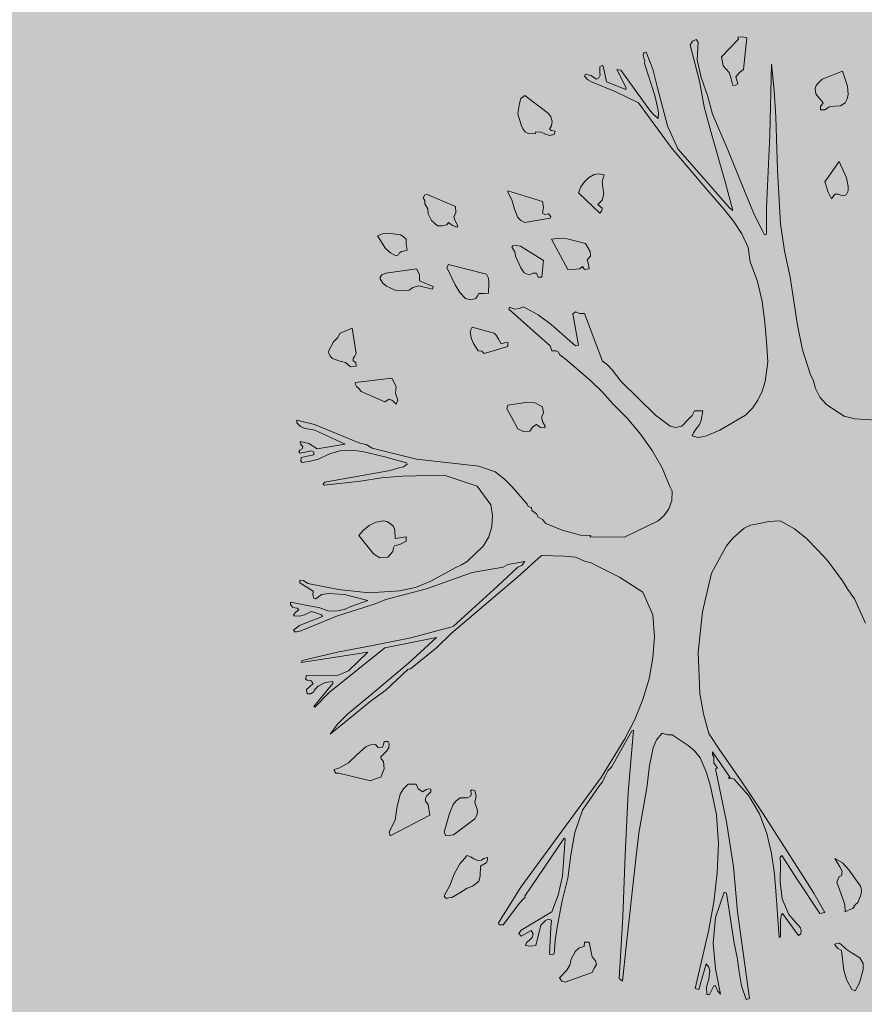
# Model space of a CAD drawing. Units: inches. Extents: x 84 to 1044, y -280 to 906.
# Tile 31 of 105: x 789 to 809, y -108 to -84. Entities that reach past the tile are written whole.
import ezdxf

# ---------------------------------------------------------------- set-up
doc = ezdxf.new("R2010")
doc.units = ezdxf.units.IN
doc.layers.add('L-PLNT', color=114, linetype='Continuous', lineweight=15)
doc.layers.add('L-PLNT-PATT', color=9, linetype='Continuous', lineweight=9, true_color=0xafd9aa)

# ---------------------------------------------------------------- blocks, each defined once
blk = doc.blocks.new('A$C37E508DF')
for p, q in [((0.6329, 1.5111), (0.6367, 1.5175)), ((0.6367, 1.5175), (0.6423, 1.5201)), ((0.6423, 1.5201), (0.6453, 1.5158)), ((0.6453, 1.5158), (0.644, 1.4879)), ((0.6826, 1.493), (0.7096, 1.5209)), ((0.7083, 1.5239), (0.7152, 1.5244)), ((0.7096, 1.5209), (0.7083, 1.5239)), ((0.7152, 1.5244), (0.7225, 1.5231)), ((0.7225, 1.5231), (0.7174, 1.4729)), ((0.5583, 1.4948), (0.5596, 1.4995)), ((0.5596, 1.4995), (0.563, 1.5003)), ((0.563, 1.5003), (0.5737, 1.4733)), ((0.6475, 1.4545), (0.6329, 1.5111)), ((0.5596, 1.4905), (0.5583, 1.4948)), ((0.5613, 1.4862), (0.5596, 1.4905)), ((0.5608, 1.4823), (0.5613, 1.4862)), ((0.5767, 1.4317), (0.5608, 1.4823)), ((0.644, 1.4879), (0.6505, 1.46)), ((0.6852, 1.4785), (0.6826, 1.493)), ((0.4897, 1.4772), (0.4935, 1.4789)), ((0.4897, 1.4678), (0.4897, 1.4772)), ((0.4905, 1.4635), (0.4897, 1.4678)), ((0.4935, 1.4789), (0.4952, 1.478)), ((0.4952, 1.478), (0.5004, 1.4532)), ((0.5313, 1.4437), (0.5167, 1.4729)), ((0.5167, 1.4729), (0.5231, 1.4716)), ((0.5231, 1.4716), (0.5686, 1.409)), ((0.5737, 1.4733), (0.5814, 1.4437)), ((0.6946, 1.4682), (0.6852, 1.4785)), ((0.6976, 1.4579), (0.6946, 1.4682)), ((0.7109, 1.4682), (0.7053, 1.4609)), ((0.7174, 1.4729), (0.7109, 1.4682)), ((0.7589, 1.3691), (0.7615, 1.481)), ((0.7615, 1.481), (0.7658, 1.4395)), ((0.8421, 1.4575), (0.8739, 1.4703)), ((0.8739, 1.4703), (0.882, 1.4463)), ((0.4657, 1.4622), (0.4669, 1.4652)), ((0.4708, 1.4566), (0.4657, 1.4622)), ((0.4669, 1.4652), (0.4755, 1.463)), ((0.4764, 1.4532), (0.4708, 1.4566)), ((0.4755, 1.463), (0.4845, 1.4575)), ((0.5154, 1.4373), (0.4764, 1.4532)), ((0.4845, 1.4575), (0.4884, 1.4596)), ((0.4884, 1.4596), (0.4905, 1.4635)), ((0.5004, 1.4532), (0.5308, 1.4412)), ((0.6552, 1.4137), (0.6475, 1.4545)), ((0.6505, 1.46), (0.6603, 1.4317)), ((0.7002, 1.4476), (0.6976, 1.4579)), ((0.7053, 1.4609), (0.7083, 1.4502)), ((0.8323, 1.4476), (0.8357, 1.451)), ((0.8357, 1.451), (0.8421, 1.4575)), ((0.551, 1.4197), (0.5154, 1.4373)), ((0.5308, 1.4412), (0.5313, 1.4437)), ((0.5814, 1.4437), (0.5969, 1.3833)), ((0.7049, 1.448), (0.7002, 1.4476)), ((0.7083, 1.4502), (0.7049, 1.448)), ((0.7658, 1.4395), (0.7684, 1.3979)), ((0.831, 1.4424), (0.8323, 1.4476)), ((0.8318, 1.4343), (0.831, 1.4424)), ((0.882, 1.4463), (0.8829, 1.433)), ((0.3628, 1.4189), (0.3649, 1.4266)), ((0.3649, 1.4266), (0.3709, 1.4317)), ((0.3709, 1.4317), (0.4086, 1.403)), ((0.6029, 1.3494), (0.551, 1.4197)), ((0.5814, 1.4133), (0.5767, 1.4317)), ((0.6603, 1.4317), (0.668, 1.4021)), ((0.8353, 1.4292), (0.8318, 1.4343)), ((0.8434, 1.4197), (0.8353, 1.4292)), ((0.8391, 1.4141), (0.8434, 1.4197)), ((0.8781, 1.4197), (0.8709, 1.4154)), ((0.8816, 1.4262), (0.8781, 1.4197)), ((0.8829, 1.433), (0.8816, 1.4262)), ((0.3598, 1.403), (0.3628, 1.4189)), ((0.5686, 1.409), (0.5741, 1.4021)), ((0.5827, 1.4043), (0.5814, 1.4133)), ((0.5823, 1.3953), (0.5827, 1.4043)), ((0.6655, 1.3743), (0.6552, 1.4137)), ((0.8395, 1.4086), (0.8391, 1.4141)), ((0.846, 1.4086), (0.8395, 1.4086)), ((0.8528, 1.4137), (0.846, 1.4086)), ((0.8619, 1.4146), (0.8528, 1.4137)), ((0.8709, 1.4154), (0.8619, 1.4146)), ((0.3602, 1.4021), (0.3598, 1.403)), ((0.364, 1.3888), (0.3602, 1.4021)), ((0.3657, 1.3828), (0.364, 1.3888)), ((0.4086, 1.403), (0.4125, 1.3979)), ((0.4125, 1.3979), (0.4142, 1.391)), ((0.4142, 1.391), (0.4134, 1.3837)), ((0.5741, 1.4021), (0.5823, 1.3953)), ((0.668, 1.4021), (0.6925, 1.3455)), ((0.7684, 1.3979), (0.771, 1.3134)), ((0.3683, 1.3781), (0.3657, 1.3828)), ((0.3718, 1.3738), (0.3683, 1.3781)), ((0.3765, 1.3713), (0.3718, 1.3738)), ((0.3885, 1.3738), (0.3872, 1.3708)), ((0.3971, 1.3734), (0.3885, 1.3738)), ((0.4039, 1.3704), (0.3971, 1.3734)), ((0.4134, 1.3837), (0.4099, 1.3781)), ((0.4099, 1.3781), (0.4134, 1.376)), ((0.4134, 1.376), (0.4189, 1.3751)), ((0.4189, 1.3751), (0.4176, 1.37)), ((0.5969, 1.3833), (0.6132, 1.3472)), ((0.6882, 1.2949), (0.6655, 1.3743)), ((0.3872, 1.3708), (0.3765, 1.3713)), ((0.4108, 1.3683), (0.4039, 1.3704)), ((0.4176, 1.37), (0.4108, 1.3683)), ((0.7538, 1.2529), (0.7589, 1.3691)), ((0.6595, 1.2829), (0.6029, 1.3494)), ((0.6132, 1.3472), (0.6959, 1.2529)), ((0.6925, 1.3455), (0.7161, 1.2868)), ((0.846, 1.2949), (0.8687, 1.3271)), ((0.8687, 1.3271), (0.8803, 1.3014)), ((0.771, 1.3134), (0.7761, 1.2285)), ((0.4597, 1.2868), (0.4648, 1.2945)), ((0.4648, 1.2945), (0.4717, 1.3009)), ((0.4717, 1.3009), (0.4807, 1.3065)), ((0.4807, 1.3065), (0.4884, 1.3074)), ((0.4884, 1.3074), (0.4965, 1.3057)), ((0.4965, 1.3057), (0.4935, 1.2954)), ((0.4935, 1.2954), (0.4948, 1.2855)), ((0.7002, 1.2495), (0.6882, 1.2949)), ((0.8473, 1.2924), (0.846, 1.2949)), ((0.8803, 1.3014), (0.8833, 1.2872)), ((0.3439, 1.2804), (0.3992, 1.2636)), ((0.3439, 1.2787), (0.3439, 1.2804)), ((0.4562, 1.2774), (0.4597, 1.2868)), ((0.4948, 1.2855), (0.4961, 1.2756)), ((0.6865, 1.2508), (0.6595, 1.2829)), ((0.7161, 1.2868), (0.7349, 1.2422)), ((0.8507, 1.2795), (0.8473, 1.2924)), ((0.8567, 1.2679), (0.8507, 1.2795)), ((0.8829, 1.2808), (0.8799, 1.2744)), ((0.8833, 1.2872), (0.8829, 1.2808)), ((0.2101, 1.2696), (0.2127, 1.2744)), ((0.2127, 1.2654), (0.2101, 1.2696)), ((0.2127, 1.2744), (0.2152, 1.2752)), ((0.2127, 1.2602), (0.2127, 1.2654)), ((0.2152, 1.2752), (0.2611, 1.2559)), ((0.3507, 1.2662), (0.3439, 1.2787)), ((0.3546, 1.2516), (0.3507, 1.2662)), ((0.3992, 1.2636), (0.4005, 1.2546)), ((0.4897, 1.2452), (0.4562, 1.2774)), ((0.4935, 1.2658), (0.4867, 1.2589)), ((0.4961, 1.2756), (0.4935, 1.2658)), ((0.8619, 1.2752), (0.8567, 1.2679)), ((0.867, 1.2752), (0.8619, 1.2752)), ((0.8713, 1.2739), (0.867, 1.2752)), ((0.8756, 1.2726), (0.8713, 1.2739)), ((0.8799, 1.2744), (0.8756, 1.2726)), ((0.2174, 1.2521), (0.2127, 1.2602)), ((0.2182, 1.2443), (0.2174, 1.2521)), ((0.2611, 1.2559), (0.262, 1.2465)), ((0.3602, 1.2383), (0.3546, 1.2516)), ((0.4005, 1.2546), (0.3992, 1.2452)), ((0.4867, 1.2589), (0.4935, 1.2529)), ((0.4931, 1.2491), (0.4897, 1.2452)), ((0.4935, 1.2529), (0.4931, 1.2491)), ((0.7015, 1.2323), (0.6865, 1.2508)), ((0.6959, 1.2529), (0.7002, 1.2495)), ((0.7538, 1.2122), (0.7538, 1.2529)), ((0.2234, 1.2336), (0.2182, 1.2443)), ((0.2328, 1.2251), (0.2234, 1.2336)), ((0.262, 1.2465), (0.2586, 1.2388)), ((0.2586, 1.2388), (0.2611, 1.2319)), ((0.3649, 1.2336), (0.3602, 1.2383)), ((0.3709, 1.2306), (0.3649, 1.2336)), ((0.4112, 1.2375), (0.3709, 1.2306)), ((0.3992, 1.2452), (0.4026, 1.2431)), ((0.4026, 1.2431), (0.4086, 1.2443)), ((0.4086, 1.2443), (0.4121, 1.2401)), ((0.4121, 1.2401), (0.4112, 1.2375)), ((0.7148, 1.2126), (0.7015, 1.2323)), ((0.7349, 1.2422), (0.7482, 1.216)), ((0.2401, 1.2251), (0.2328, 1.2251)), ((0.2474, 1.2268), (0.2401, 1.2251)), ((0.2504, 1.2306), (0.2474, 1.2268)), ((0.2568, 1.2255), (0.2504, 1.2306)), ((0.2633, 1.2229), (0.2568, 1.2255)), ((0.2611, 1.2319), (0.265, 1.2251)), ((0.265, 1.2251), (0.2633, 1.2229)), ((0.7761, 1.2285), (0.7821, 1.1856)), ((0.1376, 1.2092), (0.1458, 1.2126)), ((0.1389, 1.2079), (0.1376, 1.2092)), ((0.1505, 1.189), (0.1389, 1.2079)), ((0.1458, 1.2126), (0.1548, 1.2135)), ((0.1548, 1.2135), (0.1741, 1.2109)), ((0.1741, 1.2109), (0.1784, 1.2083)), ((0.1784, 1.2083), (0.1831, 1.204)), ((0.1831, 1.204), (0.1831, 1.1959)), ((0.4134, 1.204), (0.4258, 1.2058)), ((0.4391, 1.156), (0.4134, 1.204)), ((0.4258, 1.2058), (0.4382, 1.2045)), ((0.4382, 1.2045), (0.4669, 1.1972)), ((0.7246, 1.1908), (0.7148, 1.2126)), ((0.7482, 1.216), (0.7508, 1.2109)), ((0.7508, 1.2109), (0.7538, 1.2122)), ((0.1582, 1.1822), (0.1505, 1.189)), ((0.1788, 1.1852), (0.1758, 1.1847)), ((0.1848, 1.1865), (0.1788, 1.1852)), ((0.1831, 1.1959), (0.1848, 1.1865)), ((0.3507, 1.1916), (0.352, 1.1933)), ((0.355, 1.1839), (0.3507, 1.1916)), ((0.352, 1.1933), (0.3576, 1.1942)), ((0.3576, 1.1942), (0.364, 1.1929)), ((0.364, 1.1929), (0.4005, 1.1702)), ((0.4669, 1.1972), (0.4747, 1.1843)), ((0.7281, 1.168), (0.7246, 1.1908)), ((0.7821, 1.1856), (0.7911, 1.1436)), ((0.1668, 1.1775), (0.1582, 1.1822)), ((0.1711, 1.1792), (0.1668, 1.1775)), ((0.1728, 1.1826), (0.1711, 1.1792)), ((0.1758, 1.1847), (0.1728, 1.1826)), ((0.3563, 1.177), (0.355, 1.1839)), ((0.3645, 1.1586), (0.3563, 1.177)), ((0.4005, 1.1702), (0.3979, 1.1436)), ((0.4751, 1.177), (0.47, 1.1714)), ((0.47, 1.1714), (0.4721, 1.1646)), ((0.4747, 1.1843), (0.4751, 1.177)), ((0.1509, 1.1504), (0.1994, 1.1573)), ((0.1994, 1.1573), (0.2041, 1.1479)), ((0.2478, 1.1594), (0.2504, 1.1637)), ((0.2607, 1.1316), (0.2478, 1.1594)), ((0.2504, 1.1637), (0.3104, 1.1487)), ((0.37, 1.1509), (0.3645, 1.1586)), ((0.4519, 1.1564), (0.4391, 1.156)), ((0.458, 1.1573), (0.4519, 1.1564)), ((0.4622, 1.1607), (0.458, 1.1573)), ((0.4657, 1.156), (0.4622, 1.1607)), ((0.473, 1.1573), (0.4657, 1.156)), ((0.4721, 1.1646), (0.473, 1.1573)), ((0.7396, 1.1371), (0.7281, 1.168)), ((0.1419, 1.1436), (0.1449, 1.1474)), ((0.1419, 1.141), (0.1419, 1.1436)), ((0.1462, 1.1342), (0.1419, 1.141)), ((0.1449, 1.1474), (0.1509, 1.1504)), ((0.2041, 1.1479), (0.2045, 1.138)), ((0.3104, 1.1487), (0.3134, 1.1423)), ((0.3134, 1.1423), (0.3139, 1.1346)), ((0.3778, 1.1474), (0.37, 1.1509)), ((0.3842, 1.15), (0.3778, 1.1474)), ((0.3898, 1.15), (0.3842, 1.15)), ((0.3923, 1.1436), (0.3898, 1.15)), ((0.3979, 1.1436), (0.3923, 1.1436)), ((0.7911, 1.1436), (0.8027, 1.0677)), ((0.1522, 1.1294), (0.1462, 1.1342)), ((0.1655, 1.1234), (0.1522, 1.1294)), ((0.181, 1.1226), (0.1655, 1.1234)), ((0.1878, 1.1234), (0.181, 1.1226)), ((0.1938, 1.1273), (0.1878, 1.1234)), ((0.2032, 1.1303), (0.1938, 1.1273)), ((0.2247, 1.1251), (0.2032, 1.1303)), ((0.2045, 1.138), (0.226, 1.129)), ((0.226, 1.129), (0.2247, 1.1251)), ((0.268, 1.1196), (0.2607, 1.1316)), ((0.3139, 1.1346), (0.3134, 1.1183)), ((0.7469, 1.1054), (0.7396, 1.1371)), ((0.277, 1.1101), (0.268, 1.1196)), ((0.2856, 1.108), (0.277, 1.1101)), ((0.2933, 1.1101), (0.2856, 1.108)), ((0.2959, 1.1144), (0.2933, 1.1101)), ((0.2984, 1.1179), (0.2959, 1.1144)), ((0.3066, 1.1179), (0.2984, 1.1179)), ((0.3134, 1.1183), (0.3066, 1.1179)), ((0.3456, 1.093), (0.3469, 1.0964)), ((0.3842, 1.0591), (0.3456, 1.093)), ((0.3469, 1.0964), (0.355, 1.093)), ((0.355, 1.093), (0.3619, 1.0943)), ((0.3619, 1.0943), (0.3692, 1.0968)), ((0.3692, 1.0968), (0.3923, 1.0844)), ((0.7512, 1.0728), (0.7469, 1.1054)), ((0.3923, 1.0844), (0.4129, 1.069)), ((0.4472, 1.0857), (0.4515, 1.0887)), ((0.4562, 1.0364), (0.4472, 1.0857)), ((0.4515, 1.0887), (0.4584, 1.0865)), ((0.4584, 1.0865), (0.4657, 1.0861)), ((0.4657, 1.0861), (0.4939, 1.0107)), ((0.0789, 1.0552), (0.0978, 1.063)), ((0.0978, 1.063), (0.1042, 1.0231)), ((0.2847, 1.0565), (0.2856, 1.0604)), ((0.2856, 1.0604), (0.2877, 1.0647)), ((0.2877, 1.0647), (0.3224, 1.0552)), ((0.4129, 1.069), (0.4515, 1.0351)), ((0.7538, 1.0415), (0.7512, 1.0728)), ((0.8027, 1.0677), (0.8108, 1.0287)), ((0.0682, 1.0415), (0.0746, 1.0475)), ((0.0746, 1.0475), (0.0789, 1.0552)), ((0.2851, 1.054), (0.2847, 1.0565)), ((0.2864, 1.0463), (0.2851, 1.054)), ((0.2899, 1.039), (0.2864, 1.0463)), ((0.3224, 1.0552), (0.3255, 1.0522)), ((0.3255, 1.0522), (0.3293, 1.0458)), ((0.3293, 1.0458), (0.3336, 1.0381)), ((0.4112, 1.0351), (0.3842, 1.0591)), ((0.0596, 1.0257), (0.0682, 1.0415)), ((0.2972, 1.0274), (0.2899, 1.039)), ((0.3439, 1.0338), (0.3066, 1.0231)), ((0.3336, 1.0381), (0.3383, 1.0398)), ((0.3383, 1.0398), (0.3439, 1.0402)), ((0.3439, 1.0402), (0.3439, 1.0338)), ((0.4138, 1.0274), (0.4112, 1.0351)), ((0.4515, 1.0351), (0.4562, 1.0364)), ((0.7559, 1.0098), (0.7538, 1.0415)), ((0.0626, 1.0188), (0.0596, 1.0257)), ((0.0665, 1.0149), (0.0626, 1.0188)), ((0.0763, 1.0111), (0.0665, 1.0149)), ((0.1012, 1.018), (0.099, 1.0149)), ((0.099, 1.0149), (0.099, 1.0111)), ((0.1042, 1.0231), (0.1012, 1.018)), ((0.3032, 1.0265), (0.2972, 1.0274)), ((0.3066, 1.0231), (0.3032, 1.0265)), ((0.4202, 1.0274), (0.4138, 1.0274)), ((0.4241, 1.0257), (0.4202, 1.0274)), ((0.4267, 1.0209), (0.4241, 1.0257)), ((0.4305, 1.0175), (0.4267, 1.0209)), ((0.4378, 1.0124), (0.4305, 1.0175)), ((0.8108, 1.0287), (0.8233, 0.9892)), ((0.087, 1.0085), (0.0763, 1.0111)), ((0.0948, 1.0016), (0.087, 1.0085)), ((0.1042, 1.0029), (0.0948, 1.0016)), ((0.099, 1.0111), (0.1033, 1.0085)), ((0.1033, 1.0085), (0.1042, 1.0029)), ((0.476, 0.9789), (0.4378, 1.0124)), ((0.4939, 1.0107), (0.5021, 1.0051)), ((0.5021, 1.0051), (0.5094, 0.9969)), ((0.7516, 0.9785), (0.7559, 1.0098)), ((0.1029, 0.9772), (0.1604, 0.9841)), ((0.1604, 0.9841), (0.1672, 0.9708)), ((0.5094, 0.9969), (0.5231, 0.9789)), ((0.8233, 0.9892), (0.8275, 0.9815)), ((0.1025, 0.9751), (0.1029, 0.9772)), ((0.1046, 0.9708), (0.1025, 0.9751)), ((0.1076, 0.9682), (0.1046, 0.9708)), ((0.1119, 0.9626), (0.1076, 0.9682)), ((0.1672, 0.9708), (0.1664, 0.9601)), ((0.4939, 0.9618), (0.476, 0.9789)), ((0.5231, 0.9789), (0.578, 0.9253)), ((0.7469, 0.9635), (0.7516, 0.9785)), ((0.8275, 0.9815), (0.8314, 0.9673)), ((0.8314, 0.9673), (0.8383, 0.954)), ((0.1496, 0.9463), (0.1119, 0.9626)), ((0.1664, 0.9601), (0.1698, 0.9493)), ((0.5111, 0.9429), (0.4939, 0.9618)), ((0.7401, 0.9493), (0.7469, 0.9635)), ((0.8383, 0.954), (0.8486, 0.942)), ((0.1565, 0.9506), (0.1496, 0.9463)), ((0.1604, 0.9493), (0.1565, 0.9506)), ((0.1629, 0.9468), (0.1604, 0.9493)), ((0.1672, 0.9429), (0.1629, 0.9468)), ((0.1698, 0.9493), (0.1672, 0.9429)), ((0.3426, 0.936), (0.3443, 0.9412)), ((0.3602, 0.9039), (0.3426, 0.936)), ((0.3443, 0.9412), (0.3722, 0.9451)), ((0.3722, 0.9451), (0.3868, 0.9446)), ((0.3868, 0.9446), (0.3992, 0.9386)), ((0.3992, 0.9386), (0.4009, 0.9292)), ((0.5334, 0.9202), (0.5111, 0.9429)), ((0.7203, 0.9253), (0.7315, 0.9365)), ((0.7315, 0.9365), (0.7401, 0.9493)), ((0.8486, 0.942), (0.8619, 0.933)), ((0.4009, 0.9292), (0.3975, 0.9215)), ((0.3975, 0.9215), (0.3996, 0.9142)), ((0.554, 0.8953), (0.5334, 0.9202)), ((0.578, 0.9253), (0.6011, 0.9077)), ((0.6303, 0.9189), (0.6359, 0.9245)), ((0.6359, 0.9245), (0.6397, 0.9322)), ((0.6397, 0.9322), (0.653, 0.9322)), ((0.653, 0.9322), (0.6505, 0.9172)), ((0.6796, 0.9013), (0.7203, 0.9253)), ((0.8619, 0.933), (0.8769, 0.9236)), ((0.8769, 0.9236), (0.8936, 0.9193)), ((0.0103, 0.9129), (0.0103, 0.9172)), ((0.0103, 0.9172), (0.0382, 0.9107)), ((0.0159, 0.9073), (0.0103, 0.9129)), ((0.0232, 0.9043), (0.0159, 0.9073)), ((0.0382, 0.9107), (0.1098, 0.8807)), ((0.3838, 0.9069), (0.379, 0.9)), ((0.3898, 0.9107), (0.3838, 0.9069)), ((0.3958, 0.906), (0.3898, 0.9107)), ((0.4026, 0.9052), (0.3958, 0.906)), ((0.3996, 0.9142), (0.4031, 0.9077)), ((0.4031, 0.9077), (0.4026, 0.9052)), ((0.6011, 0.9077), (0.6097, 0.9056)), ((0.6097, 0.9056), (0.6196, 0.9077)), ((0.6196, 0.9077), (0.6303, 0.9189)), ((0.6479, 0.9103), (0.6423, 0.9039)), ((0.6505, 0.9172), (0.6479, 0.9103)), ((0.8936, 0.9193), (0.9279, 0.9172)), ((0.0386, 0.9013), (0.0232, 0.9043)), ((0.0866, 0.8794), (0.0386, 0.9013)), ((0.3692, 0.8992), (0.3602, 0.9039)), ((0.379, 0.9), (0.3692, 0.8992)), ((0.5728, 0.8691), (0.554, 0.8953)), ((0.6384, 0.8974), (0.6359, 0.8927)), ((0.6359, 0.8927), (0.6457, 0.8897)), ((0.6423, 0.9039), (0.6384, 0.8974)), ((0.6457, 0.8897), (0.6569, 0.8919)), ((0.6569, 0.8919), (0.6796, 0.9013)), ((0.0159, 0.8803), (0.0154, 0.8837)), ((0.0154, 0.8837), (0.0292, 0.8803)), ((0.0176, 0.8777), (0.0159, 0.8803)), ((0.0193, 0.8752), (0.0176, 0.8777)), ((0.0184, 0.8717), (0.0193, 0.8752)), ((0.0292, 0.8803), (0.0424, 0.8717)), ((0.0424, 0.8717), (0.0866, 0.8794)), ((0.1098, 0.8807), (0.1196, 0.8786)), ((0.1196, 0.8786), (0.1295, 0.873)), ((0.0133, 0.8679), (0.015, 0.87)), ((0.0154, 0.8649), (0.0133, 0.8679)), ((0.015, 0.87), (0.0184, 0.8717)), ((0.0334, 0.8687), (0.0154, 0.8649)), ((0.0163, 0.8529), (0.0171, 0.8584)), ((0.0171, 0.8584), (0.0266, 0.8602)), ((0.0266, 0.8602), (0.0369, 0.8623)), ((0.0369, 0.8666), (0.0334, 0.8687)), ((0.0369, 0.8623), (0.0369, 0.8666)), ((0.0617, 0.864), (0.0442, 0.8554)), ((0.0789, 0.8687), (0.0617, 0.864)), ((0.0965, 0.8696), (0.0789, 0.8687)), ((0.1141, 0.8679), (0.0965, 0.8696)), ((0.1492, 0.8593), (0.1141, 0.8679)), ((0.1295, 0.873), (0.1994, 0.8554)), ((0.1835, 0.8499), (0.1492, 0.8593)), ((0.5887, 0.8421), (0.5728, 0.8691)), ((0.0184, 0.8503), (0.0163, 0.8529)), ((0.0317, 0.8524), (0.0184, 0.8503)), ((0.0442, 0.8554), (0.0317, 0.8524)), ((0.1698, 0.8413), (0.1792, 0.8434)), ((0.1792, 0.8434), (0.1848, 0.8477)), ((0.1848, 0.8477), (0.1835, 0.8499)), ((0.1994, 0.8554), (0.2984, 0.8447)), ((0.2984, 0.8447), (0.3242, 0.8357)), ((0.6007, 0.8125), (0.5887, 0.8421)), ((0.0545, 0.8194), (0.1578, 0.8378)), ((0.1771, 0.8288), (0.1441, 0.8258)), ((0.1578, 0.8378), (0.1698, 0.8413)), ((0.2436, 0.8301), (0.1771, 0.8288)), ((0.2954, 0.813), (0.2436, 0.8301)), ((0.3242, 0.8357), (0.3387, 0.8241)), ((0.0519, 0.8164), (0.0545, 0.8194)), ((0.0532, 0.8143), (0.0519, 0.8164)), ((0.1111, 0.8207), (0.0532, 0.8143)), ((0.1441, 0.8258), (0.1111, 0.8207)), ((0.3173, 0.7834), (0.2954, 0.813)), ((0.3387, 0.8241), (0.3512, 0.8117)), ((0.3512, 0.8117), (0.3748, 0.7842)), ((0.6046, 0.8048), (0.6007, 0.8125)), ((0.6037, 0.7903), (0.6046, 0.8048)), ((0.3199, 0.7662), (0.3173, 0.7834)), ((0.3748, 0.7842), (0.3765, 0.7804)), ((0.3765, 0.7804), (0.3816, 0.7791)), ((0.599, 0.777), (0.6037, 0.7903)), ((0.3186, 0.7491), (0.3199, 0.7662)), ((0.3816, 0.7791), (0.382, 0.7744)), ((0.382, 0.7744), (0.3859, 0.7714)), ((0.3859, 0.7714), (0.3902, 0.7684)), ((0.3902, 0.7684), (0.3919, 0.7641)), ((0.5823, 0.7577), (0.5913, 0.7658)), ((0.5913, 0.7658), (0.599, 0.777)), ((0.1153, 0.7427), (0.1244, 0.7504)), ((0.1244, 0.7504), (0.1351, 0.7559)), ((0.1351, 0.7559), (0.1471, 0.7577)), ((0.1471, 0.7577), (0.1527, 0.7568)), ((0.1527, 0.7568), (0.1578, 0.7538)), ((0.1578, 0.7538), (0.1629, 0.7491)), ((0.1629, 0.7491), (0.1651, 0.7431)), ((0.3139, 0.7324), (0.3186, 0.7491)), ((0.3919, 0.7641), (0.3988, 0.7598)), ((0.3988, 0.7598), (0.4043, 0.7538)), ((0.4043, 0.7538), (0.4301, 0.7431)), ((0.5287, 0.7319), (0.5823, 0.7577)), ((0.7285, 0.7512), (0.7182, 0.7461)), ((0.7401, 0.7534), (0.7285, 0.7512)), ((0.7577, 0.7568), (0.7401, 0.7534)), ((0.7752, 0.7577), (0.7577, 0.7568)), ((0.798, 0.7452), (0.7752, 0.7577)), ((0.1081, 0.7349), (0.1153, 0.7427)), ((0.1312, 0.7058), (0.1081, 0.7349)), ((0.1651, 0.7431), (0.1655, 0.7298)), ((0.4301, 0.7431), (0.4515, 0.7371)), ((0.4515, 0.7371), (0.4635, 0.7341)), ((0.4635, 0.7341), (0.4755, 0.7349)), ((0.4755, 0.7349), (0.4742, 0.7324)), ((0.7182, 0.7461), (0.7002, 0.7307)), ((0.8173, 0.7298), (0.798, 0.7452)), ((0.1646, 0.7186), (0.1629, 0.7152)), ((0.1741, 0.7208), (0.1646, 0.7186)), ((0.1655, 0.7298), (0.1831, 0.7324)), ((0.1831, 0.7255), (0.1741, 0.7208)), ((0.1831, 0.7324), (0.1831, 0.7255)), ((0.28, 0.6933), (0.3049, 0.7178)), ((0.3049, 0.7178), (0.3139, 0.7324)), ((0.4742, 0.7324), (0.5287, 0.7319)), ((0.6903, 0.7186), (0.6818, 0.7032)), ((0.7002, 0.7307), (0.6903, 0.7186)), ((0.8344, 0.7122), (0.8173, 0.7298)), ((0.1415, 0.6994), (0.1312, 0.7058)), ((0.1621, 0.7092), (0.1539, 0.7002)), ((0.1629, 0.7152), (0.1621, 0.7092)), ((0.3975, 0.7028), (0.3598, 0.6693)), ((0.4339, 0.7019), (0.3975, 0.7028)), ((0.4515, 0.7002), (0.4339, 0.7019)), ((0.6818, 0.7032), (0.6667, 0.6749)), ((0.8503, 0.6951), (0.8344, 0.7122)), ((0.1539, 0.7002), (0.1415, 0.6994)), ((0.262, 0.6839), (0.271, 0.6882)), ((0.271, 0.6882), (0.28, 0.6933)), ((0.3443, 0.6886), (0.337, 0.6843)), ((0.3533, 0.6903), (0.3443, 0.6886)), ((0.3709, 0.6933), (0.3533, 0.6903)), ((0.3598, 0.6843), (0.3662, 0.6873)), ((0.3662, 0.6873), (0.3709, 0.6933)), ((0.4674, 0.6933), (0.4515, 0.7002)), ((0.476, 0.6912), (0.4674, 0.6933)), ((0.4832, 0.6878), (0.476, 0.6912)), ((0.521, 0.6685), (0.4832, 0.6878)), ((0.8739, 0.6629), (0.8503, 0.6951)), ((0.2877, 0.6762), (0.2152, 0.6505)), ((0.2221, 0.6625), (0.262, 0.6839)), ((0.337, 0.6843), (0.2877, 0.6762)), ((0.328, 0.6543), (0.3598, 0.6843)), ((0.6667, 0.6749), (0.6526, 0.614)), ((0.0146, 0.6599), (0.0146, 0.6642)), ((0.0146, 0.6642), (0.0206, 0.6633)), ((0.036, 0.6466), (0.0146, 0.6599)), ((0.0206, 0.6633), (0.0274, 0.6586)), ((0.0274, 0.6586), (0.0759, 0.6492)), ((0.1977, 0.6526), (0.2221, 0.6625)), ((0.3598, 0.6693), (0.2543, 0.5797)), ((0.5578, 0.6449), (0.521, 0.6685)), ((0.8824, 0.6492), (0.8739, 0.6629)), ((0.0356, 0.6406), (0.036, 0.6466)), ((0.0369, 0.6355), (0.0356, 0.6406)), ((0.0489, 0.641), (0.0399, 0.6342)), ((0.0609, 0.6428), (0.0489, 0.641)), ((0.0853, 0.641), (0.0609, 0.6428)), ((0.0759, 0.6492), (0.1244, 0.644)), ((0.1226, 0.632), (0.0853, 0.641)), ((0.1244, 0.644), (0.1728, 0.647)), ((0.2152, 0.6505), (0.1509, 0.6333)), ((0.1728, 0.647), (0.1977, 0.6526)), ((0.2581, 0.5913), (0.328, 0.6543)), ((0.5737, 0.6089), (0.5578, 0.6449)), ((0.8932, 0.6342), (0.8824, 0.6492)), ((0, 0.629), (0.0467, 0.62)), ((0, 0.6252), (0, 0.629)), ((0.003, 0.6213), (0, 0.6252)), ((0.0399, 0.6342), (0.0369, 0.6355)), ((0.0973, 0.6226), (0.1226, 0.632)), ((0.1342, 0.6265), (0.1175, 0.6213)), ((0.1509, 0.6333), (0.1342, 0.6265)), ((0.9103, 0.5956), (0.8932, 0.6342)), ((0.0069, 0.6204), (0.003, 0.6213)), ((0.0047, 0.6093), (0.0086, 0.6132)), ((0.0056, 0.6076), (0.0047, 0.6093)), ((0.0107, 0.6196), (0.0069, 0.6204)), ((0.0086, 0.6132), (0.0133, 0.617)), ((0.0133, 0.617), (0.0107, 0.6196)), ((0.0223, 0.6089), (0.0141, 0.6072)), ((0.0334, 0.6145), (0.0223, 0.6089)), ((0.0416, 0.6119), (0.0334, 0.6145)), ((0.0493, 0.6093), (0.0416, 0.6119)), ((0.0467, 0.62), (0.0592, 0.6153)), ((0.0506, 0.6063), (0.0493, 0.6093)), ((0.0592, 0.6153), (0.072, 0.6149)), ((0.072, 0.6149), (0.0849, 0.6175)), ((0.1175, 0.6213), (0.0746, 0.6076)), ((0.0849, 0.6175), (0.0973, 0.6226)), ((0.5763, 0.5741), (0.5737, 0.6089)), ((0.6526, 0.614), (0.6457, 0.5497)), ((0.0141, 0.6072), (0.0056, 0.6076)), ((0.0141, 0.5921), (0.0257, 0.5969)), ((0.0746, 0.6076), (0.0163, 0.5836)), ((0.0257, 0.5969), (0.0506, 0.6063)), ((0.0047, 0.5849), (0.0141, 0.5921)), ((0.0069, 0.5823), (0.0047, 0.5849)), ((0.0099, 0.5823), (0.0069, 0.5823)), ((0.0163, 0.5836), (0.0099, 0.5823)), ((0.1904, 0.5724), (0.2474, 0.5879)), ((0.2543, 0.5797), (0.2311, 0.557)), ((0.2474, 0.5879), (0.253, 0.5892)), ((0.253, 0.5892), (0.2581, 0.5913)), ((0.1325, 0.5608), (0.1904, 0.5724)), ((0.2311, 0.5729), (0.1496, 0.557)), ((0.1869, 0.5325), (0.2311, 0.5729)), ((0.5737, 0.5407), (0.5763, 0.5741)), ((0.1226, 0.5497), (0.0171, 0.5338)), ((0.0184, 0.5368), (0.0746, 0.5501)), ((0.1496, 0.557), (0.0613, 0.4858)), ((0.0746, 0.5501), (0.1325, 0.5608)), ((0.0917, 0.5205), (0.1226, 0.5497)), ((0.2311, 0.557), (0.1899, 0.5235)), ((0.6457, 0.5497), (0.6483, 0.4845)), ((0.0171, 0.5338), (0.0184, 0.5368)), ((0.1269, 0.482), (0.1869, 0.5325)), ((0.5677, 0.5077), (0.5737, 0.5407)), ((0.0755, 0.5133), (0.0917, 0.5205)), ((0.1861, 0.5231), (0.1509, 0.4897)), ((0.1899, 0.5235), (0.1861, 0.5231)), ((0.024, 0.5072), (0.0253, 0.5128)), ((0.0262, 0.5055), (0.024, 0.5072)), ((0.0253, 0.5128), (0.042, 0.5133)), ((0.0326, 0.5047), (0.0262, 0.5055)), ((0.03, 0.4948), (0.036, 0.5004)), ((0.036, 0.5004), (0.0326, 0.5047)), ((0.0369, 0.4639), (0.0669, 0.5004)), ((0.042, 0.5133), (0.0587, 0.5124)), ((0.0549, 0.5021), (0.0437, 0.4961)), ((0.0669, 0.5034), (0.0549, 0.5021)), ((0.0587, 0.5124), (0.0755, 0.5133)), ((0.0669, 0.5004), (0.0669, 0.5034)), ((0.5578, 0.4751), (0.5677, 0.5077)), ((0.0253, 0.491), (0.03, 0.4948)), ((0.0262, 0.4841), (0.0253, 0.491)), ((0.0317, 0.4841), (0.0262, 0.4841)), ((0.0369, 0.4871), (0.0317, 0.4841)), ((0.0382, 0.4905), (0.0369, 0.4871)), ((0.0403, 0.4922), (0.0382, 0.4905)), ((0.0613, 0.4858), (0.0386, 0.4627)), ((0.0437, 0.4961), (0.0403, 0.4922)), ((0.1509, 0.4897), (0.1282, 0.4734)), ((0.6483, 0.4845), (0.6539, 0.4524)), ((0.1282, 0.4734), (0.0626, 0.4198)), ((0.0905, 0.4515), (0.1269, 0.482)), ((0.545, 0.4434), (0.5578, 0.4751)), ((0.0386, 0.4627), (0.0369, 0.4639)), ((0.6539, 0.4524), (0.6625, 0.4211)), ((0.0746, 0.4361), (0.0905, 0.4515)), ((0.5295, 0.4125), (0.545, 0.4434)), ((0.0626, 0.4198), (0.0746, 0.4361)), ((0.5403, 0.4254), (0.5081, 0.3679)), ((0.5347, 0.3276), (0.5433, 0.4266)), ((0.5433, 0.4266), (0.5403, 0.4254)), ((0.5887, 0.4215), (0.5797, 0.4112)), ((0.5969, 0.4189), (0.5887, 0.4215)), ((0.6625, 0.4211), (0.6796, 0.3945)), ((0.1471, 0.4035), (0.1484, 0.4082)), ((0.1484, 0.4082), (0.1548, 0.4082)), ((0.1548, 0.4082), (0.1565, 0.4052)), ((0.4922, 0.3516), (0.5295, 0.4125)), ((0.5797, 0.4112), (0.5741, 0.3983)), ((0.6046, 0.4189), (0.5969, 0.4189)), ((0.6295, 0.4022), (0.6046, 0.4189)), ((0.1055, 0.388), (0.1192, 0.4001)), ((0.1192, 0.4001), (0.1265, 0.4031)), ((0.1265, 0.4031), (0.1346, 0.4039)), ((0.1346, 0.4039), (0.1389, 0.3992)), ((0.1389, 0.3992), (0.1458, 0.3996)), ((0.1518, 0.3932), (0.1432, 0.3842)), ((0.1458, 0.3996), (0.1471, 0.4035)), ((0.1556, 0.3983), (0.1518, 0.3932)), ((0.1565, 0.4052), (0.1556, 0.3983)), ((0.5741, 0.3983), (0.5686, 0.3705)), ((0.6397, 0.3936), (0.6295, 0.4022)), ((0.6487, 0.3825), (0.6397, 0.3936)), ((0.6959, 0.352), (0.668, 0.3919)), ((0.668, 0.3919), (0.668, 0.3872)), ((0.6796, 0.3945), (0.7148, 0.3447)), ((0.0763, 0.3662), (0.0917, 0.3748)), ((0.0917, 0.3748), (0.1055, 0.388)), ((0.1432, 0.3842), (0.1436, 0.3808)), ((0.1436, 0.3808), (0.1471, 0.3769)), ((0.1471, 0.3769), (0.1484, 0.3649)), ((0.6582, 0.3602), (0.6487, 0.3825)), ((0.668, 0.3872), (0.6706, 0.3842)), ((0.6706, 0.3842), (0.6702, 0.3748)), ((0.6702, 0.3748), (0.6762, 0.3662)), ((0.069, 0.364), (0.0763, 0.3662)), ((0.069, 0.3627), (0.069, 0.364)), ((0.0716, 0.3585), (0.069, 0.3627)), ((0.1484, 0.3649), (0.1432, 0.352)), ((0.5025, 0.3619), (0.4982, 0.3537)), ((0.5081, 0.3679), (0.5025, 0.3619)), ((0.5686, 0.3705), (0.5643, 0.3349)), ((0.665, 0.3379), (0.6582, 0.3602)), ((0.6762, 0.3662), (0.6732, 0.3653)), ((0.6732, 0.3653), (0.6903, 0.2813)), ((0.0763, 0.3585), (0.0716, 0.3585)), ((0.1269, 0.3464), (0.0763, 0.3585)), ((0.1355, 0.3499), (0.1269, 0.3464)), ((0.1432, 0.352), (0.1355, 0.3499)), ((0.4065, 0.2345), (0.4922, 0.3516)), ((0.4939, 0.3447), (0.4884, 0.337)), ((0.4982, 0.3537), (0.4939, 0.3447)), ((0.6933, 0.3503), (0.6959, 0.352)), ((0.6985, 0.3503), (0.6933, 0.3503)), ((0.7023, 0.349), (0.6985, 0.3503)), ((0.7259, 0.3224), (0.7023, 0.349)), ((0.7148, 0.3447), (0.7487, 0.2937)), ((0.1737, 0.325), (0.1788, 0.3336)), ((0.1788, 0.3336), (0.1861, 0.3409)), ((0.1861, 0.3409), (0.199, 0.3409)), ((0.199, 0.3409), (0.2024, 0.3336)), ((0.2024, 0.3336), (0.2097, 0.3289)), ((0.2097, 0.3289), (0.2148, 0.3323)), ((0.2148, 0.3323), (0.2182, 0.3336)), ((0.2221, 0.3289), (0.2161, 0.3224)), ((0.2182, 0.3336), (0.2221, 0.3327)), ((0.2221, 0.3327), (0.2221, 0.3289)), ((0.2851, 0.3302), (0.2877, 0.3319)), ((0.2864, 0.325), (0.2851, 0.3302)), ((0.2877, 0.3319), (0.292, 0.3306)), ((0.292, 0.3306), (0.2941, 0.322)), ((0.4884, 0.337), (0.4622, 0.2997)), ((0.53, 0.229), (0.5347, 0.3276)), ((0.5643, 0.3349), (0.5578, 0.2993)), ((0.6745, 0.2924), (0.665, 0.3379)), ((0.1689, 0.3053), (0.1737, 0.325)), ((0.2161, 0.3224), (0.214, 0.3186)), ((0.214, 0.3186), (0.214, 0.3139)), ((0.214, 0.3139), (0.2182, 0.3087)), ((0.2577, 0.3087), (0.2624, 0.3147)), ((0.2624, 0.3147), (0.2689, 0.3194)), ((0.2689, 0.3194), (0.2796, 0.3194)), ((0.2796, 0.3194), (0.2847, 0.3211)), ((0.2847, 0.3211), (0.2864, 0.325)), ((0.2941, 0.322), (0.292, 0.3117)), ((0.7427, 0.2937), (0.7259, 0.3224)), ((0.1655, 0.2843), (0.1689, 0.3053)), ((0.2182, 0.3087), (0.2204, 0.292)), ((0.2517, 0.2946), (0.2577, 0.3087)), ((0.292, 0.3117), (0.2959, 0.2993)), ((0.2959, 0.2993), (0.2954, 0.2928)), ((0.4622, 0.2997), (0.4502, 0.2645)), ((0.5578, 0.2993), (0.5518, 0.2633)), ((0.1565, 0.265), (0.1655, 0.2843)), ((0.2204, 0.292), (0.1578, 0.259)), ((0.2436, 0.265), (0.2517, 0.2946)), ((0.292, 0.286), (0.2581, 0.2607)), ((0.2954, 0.2928), (0.292, 0.286)), ((0.6775, 0.2465), (0.6745, 0.2924)), ((0.6903, 0.2813), (0.7015, 0.2101)), ((0.7542, 0.2628), (0.7427, 0.2937)), ((0.7487, 0.2937), (0.8151, 0.1899)), ((0.1578, 0.259), (0.1565, 0.265)), ((0.2461, 0.259), (0.2436, 0.265)), ((0.2581, 0.2607), (0.2461, 0.259)), ((0.4335, 0.2556), (0.3709, 0.1634)), ((0.4305, 0.1951), (0.4352, 0.2543)), ((0.4352, 0.2543), (0.4335, 0.2556)), ((0.4502, 0.2645), (0.4438, 0.2285)), ((0.5518, 0.2633), (0.5475, 0.2268)), ((0.7615, 0.2311), (0.7542, 0.2628)), ((0.3649, 0.1775), (0.4065, 0.2345)), ((0.6758, 0.2002), (0.6775, 0.2465)), ((0.268, 0.2148), (0.28, 0.2277)), ((0.28, 0.2277), (0.2851, 0.226)), ((0.2851, 0.226), (0.2903, 0.2225)), ((0.2903, 0.2225), (0.2963, 0.22)), ((0.2963, 0.22), (0.3027, 0.2204)), ((0.3027, 0.2204), (0.3061, 0.2234)), ((0.3061, 0.2234), (0.3122, 0.2247)), ((0.3122, 0.22), (0.3096, 0.2165)), ((0.3122, 0.2247), (0.3122, 0.22)), ((0.4438, 0.2285), (0.4391, 0.1921)), ((0.5261, 0.1308), (0.53, 0.229)), ((0.5475, 0.2268), (0.5313, 0.084)), ((0.7662, 0.1981), (0.7615, 0.2311)), ((0.7778, 0.2277), (0.7752, 0.2255)), ((0.7752, 0.2255), (0.7761, 0.2152)), ((0.8018, 0.1912), (0.7778, 0.2277)), ((0.8619, 0.2234), (0.8739, 0.2161)), ((0.87, 0.2101), (0.8619, 0.2234)), ((0.2594, 0.1981), (0.268, 0.2148)), ((0.301, 0.211), (0.3002, 0.1951)), ((0.3096, 0.2165), (0.301, 0.211)), ((0.7015, 0.2101), (0.7079, 0.1389)), ((0.7761, 0.2152), (0.7752, 0.1861)), ((0.8734, 0.2032), (0.87, 0.2101)), ((0.8726, 0.1955), (0.8734, 0.2032)), ((0.8739, 0.2161), (0.8841, 0.2054)), ((0.8841, 0.2054), (0.9026, 0.1792)), ((0.2521, 0.1805), (0.2594, 0.1981)), ((0.298, 0.1874), (0.292, 0.1818)), ((0.3002, 0.1951), (0.298, 0.1874)), ((0.4241, 0.1651), (0.4305, 0.1951)), ((0.4391, 0.1921), (0.4301, 0.1561)), ((0.6706, 0.1539), (0.6758, 0.2002)), ((0.7688, 0.1646), (0.7662, 0.1981)), ((0.8383, 0.1359), (0.8018, 0.1912)), ((0.8151, 0.1899), (0.8288, 0.1685)), ((0.8649, 0.1857), (0.8687, 0.1947)), ((0.8687, 0.1947), (0.8726, 0.1955)), ((0.2436, 0.1642), (0.2521, 0.1805)), ((0.28, 0.1762), (0.2684, 0.1689)), ((0.2873, 0.1788), (0.28, 0.1762)), ((0.292, 0.1818), (0.2873, 0.1788)), ((0.3293, 0.1213), (0.3649, 0.1775)), ((0.7752, 0.1861), (0.7787, 0.1591)), ((0.8743, 0.1608), (0.8649, 0.1857)), ((0.9026, 0.1792), (0.9043, 0.1732)), ((0.9043, 0.1732), (0.9035, 0.1668)), ((0.2448, 0.1616), (0.2436, 0.1642)), ((0.2478, 0.1599), (0.2448, 0.1616)), ((0.2508, 0.1608), (0.2478, 0.1599)), ((0.2556, 0.1616), (0.2508, 0.1608)), ((0.2684, 0.1689), (0.2556, 0.1616)), ((0.3692, 0.1591), (0.3628, 0.1526)), ((0.3718, 0.1616), (0.3692, 0.1591)), ((0.3709, 0.1634), (0.3718, 0.1616)), ((0.4138, 0.1389), (0.4241, 0.1651)), ((0.4301, 0.1561), (0.4224, 0.1145)), ((0.6865, 0.1698), (0.6732, 0.1295)), ((0.6903, 0.1681), (0.6865, 0.1698)), ((0.7023, 0.0892), (0.6903, 0.1681)), ((0.774, 0.0982), (0.7688, 0.1646)), ((0.7787, 0.1591), (0.789, 0.1346)), ((0.8288, 0.1685), (0.846, 0.1376)), ((0.8777, 0.1496), (0.8743, 0.1608)), ((0.9035, 0.1668), (0.8983, 0.1535)), ((0.3628, 0.1526), (0.337, 0.1183)), ((0.662, 0.108), (0.6706, 0.1539)), ((0.8781, 0.1389), (0.8777, 0.1496)), ((0.8846, 0.1419), (0.8781, 0.1389)), ((0.8902, 0.1441), (0.8846, 0.1419)), ((0.894, 0.1496), (0.8902, 0.1441)), ((0.8983, 0.1535), (0.894, 0.1496)), ((0.3653, 0.1098), (0.4138, 0.1389)), ((0.4039, 0.1248), (0.3962, 0.1175)), ((0.4082, 0.1269), (0.4039, 0.1248)), ((0.4134, 0.1256), (0.4082, 0.1269)), ((0.4121, 0.1145), (0.4134, 0.1256)), ((0.5205, 0.033), (0.5261, 0.1308)), ((0.6732, 0.1295), (0.6693, 0.0892)), ((0.7079, 0.1389), (0.7268, 0.0013)), ((0.7774, 0.1346), (0.7757, 0.1261)), ((0.7757, 0.1261), (0.7761, 0.117)), ((0.7791, 0.1359), (0.7774, 0.1346)), ((0.8044, 0.1012), (0.7791, 0.1359)), ((0.789, 0.1346), (0.8074, 0.1132)), ((0.846, 0.1376), (0.8383, 0.1359)), ((0.3306, 0.1183), (0.3293, 0.1213)), ((0.337, 0.1183), (0.3306, 0.1183)), ((0.3615, 0.1042), (0.3653, 0.1098)), ((0.3962, 0.1175), (0.3885, 0.0853)), ((0.4099, 0.0716), (0.4121, 0.1145)), ((0.4224, 0.1145), (0.4189, 0.093)), ((0.7761, 0.117), (0.7761, 0.099)), ((0.8074, 0.1132), (0.8087, 0.1089)), ((0.3653, 0.0999), (0.3615, 0.1042)), ((0.3812, 0.1089), (0.3653, 0.0999)), ((0.3782, 0.0935), (0.3825, 0.0978)), ((0.3842, 0.1037), (0.3812, 0.1089)), ((0.3825, 0.0978), (0.3842, 0.1037)), ((0.641, 0.0172), (0.662, 0.108)), ((0.7761, 0.099), (0.774, 0.0982)), ((0.8083, 0.1037), (0.8044, 0.1012)), ((0.8087, 0.1089), (0.8083, 0.1037)), ((0.3722, 0.0853), (0.3739, 0.09)), ((0.3808, 0.0845), (0.3722, 0.0853)), ((0.3739, 0.09), (0.3782, 0.0935)), ((0.3885, 0.0853), (0.3808, 0.0845)), ((0.4189, 0.093), (0.4176, 0.072)), ((0.4515, 0.0763), (0.4571, 0.0815)), ((0.4571, 0.0815), (0.4648, 0.084)), ((0.4648, 0.084), (0.4657, 0.0905)), ((0.4657, 0.0905), (0.473, 0.0905)), ((0.473, 0.0905), (0.476, 0.0746)), ((0.5313, 0.084), (0.5257, 0.0291)), ((0.6693, 0.0892), (0.6728, 0.0484)), ((0.7075, 0.0665), (0.7023, 0.0892)), ((0.8619, 0.0875), (0.8649, 0.0887)), ((0.8619, 0.0866), (0.8619, 0.0875)), ((0.8666, 0.0806), (0.8619, 0.0866)), ((0.8649, 0.0887), (0.8691, 0.0892)), ((0.8726, 0.0776), (0.8666, 0.0806)), ((0.8691, 0.0892), (0.8769, 0.0827)), ((0.8769, 0.0827), (0.8799, 0.0797)), ((0.8799, 0.0797), (0.8893, 0.0733)), ((0.4142, 0.0707), (0.4099, 0.0716)), ((0.4176, 0.072), (0.4142, 0.0707)), ((0.4425, 0.0544), (0.4442, 0.0639)), ((0.4442, 0.0639), (0.4515, 0.0763)), ((0.476, 0.0746), (0.4777, 0.0673)), ((0.4777, 0.0673), (0.4832, 0.0613)), ((0.7105, 0.0437), (0.7075, 0.0665)), ((0.8764, 0.0459), (0.8726, 0.0776)), ((0.8893, 0.0733), (0.9013, 0.066)), ((0.9013, 0.066), (0.9069, 0.057)), ((0.4378, 0.0463), (0.4425, 0.0544)), ((0.4811, 0.0493), (0.4777, 0.0424)), ((0.4845, 0.0553), (0.4811, 0.0493)), ((0.4832, 0.0613), (0.4845, 0.0553)), ((0.6582, 0.0562), (0.6466, 0.0159)), ((0.6625, 0.051), (0.6582, 0.0562)), ((0.6642, 0.045), (0.6625, 0.051)), ((0.6728, 0.0484), (0.6809, 0.0082)), ((0.9069, 0.0471), (0.9009, 0.0261)), ((0.9069, 0.057), (0.9069, 0.0471)), ((0.4258, 0.0339), (0.4378, 0.0463)), ((0.4296, 0.0291), (0.4258, 0.0339)), ((0.4777, 0.0424), (0.4348, 0.0274)), ((0.5257, 0.0291), (0.5205, 0.033)), ((0.659, 0.0193), (0.6625, 0.0321)), ((0.6625, 0.0321), (0.6642, 0.045)), ((0.7144, 0.0214), (0.7105, 0.0437)), ((0.8807, 0.0304), (0.8764, 0.0459)), ((0.4348, 0.0274), (0.4296, 0.0291)), ((0.6466, 0.0159), (0.641, 0.0172)), ((0.6595, 0.0077), (0.659, 0.0193)), ((0.6702, 0.0214), (0.6637, 0.0077)), ((0.6732, 0.0214), (0.6702, 0.0214)), ((0.6766, 0.0133), (0.6732, 0.0214)), ((0.7216, 0), (0.7144, 0.0214)), ((0.8889, 0.0159), (0.8807, 0.0304)), ((0.894, 0.0137), (0.8889, 0.0159)), ((0.9009, 0.0261), (0.894, 0.0137)), ((0.6637, 0.0077), (0.6595, 0.0077)), ((0.6809, 0.0082), (0.6766, 0.0133)), ((0.7268, 0.0013), (0.7216, 0))]:
    blk.add_line(p, q)

msp = doc.modelspace()

# ---------------------------------------------------------------- hatches: boundary and pattern name
at = {"layer": 'L-PLNT-PATT', "transparency": 33554597}
h = msp.add_hatch(color=256, dxfattribs=at)
h.dxf.hatch_style = 1
h.paths.add_polyline_path([(791.074, 31.12), (791.074, 91.12), (743.074, 91.12), (674.074, 91.12), (674.074, 31.12), (650.074, 31.12), (650.074, -112.88), (983.074, -112.88), (983.074, -64.88), (791.074, -64.88)])

# ---------------------------------------------------------------- block references
at = {"layer": 'L-PLNT', "xscale": 15.19586232982809, "yscale": 15.19586232982809, "zscale": 15.19586232982809}
msp.add_blockref('A$C37E508DF', (795.564, -107.745), dxfattribs=at)

doc.saveas('drawing.dxf')
